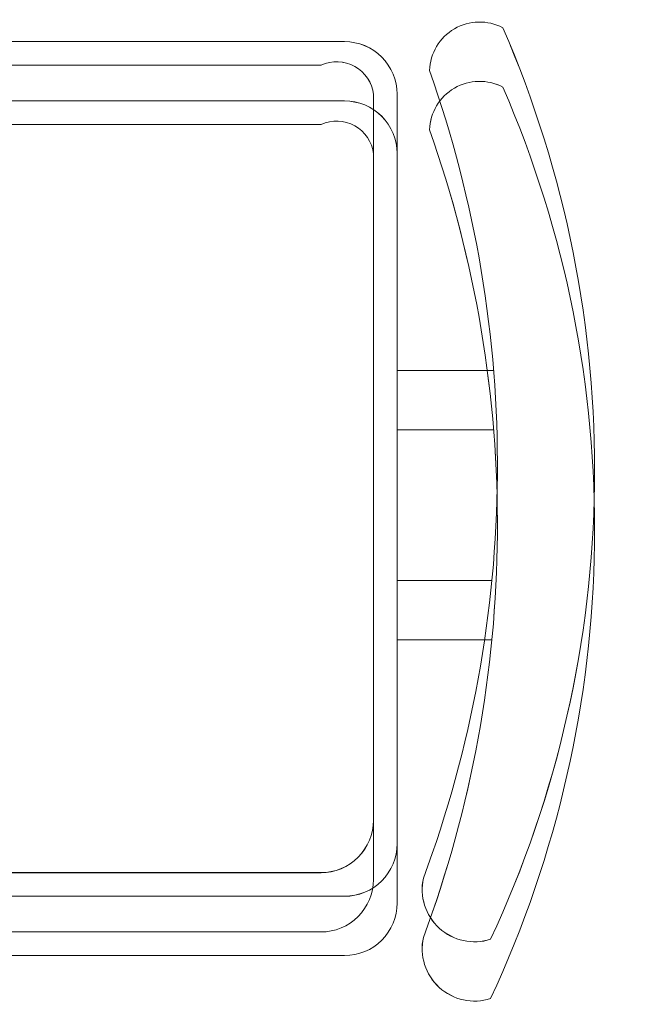
# Model space of a CAD drawing. Units: inches. Extents: x 1885 to 2748, y 783 to 2421.
# Tile 84 of 117: x 2175.64 to 2183.41, y 2082.31 to 2094.85. Entities that reach past the tile are written whole.
import ezdxf

# ---------------------------------------------------------------- set-up
doc = ezdxf.new("R2010")
doc.units = ezdxf.units.IN
doc.layers.add('A-FURN', color=8, linetype='Continuous', lineweight=13)

# ---------------------------------------------------------------- blocks, each defined once
blk = doc.blocks.new('CHAIR-DINING-END')
for points in [[(10.534, 11.861, -0.175809), (10.456, 1.571, 0.578392), (11.313, 0.792, 0.214524), (11.469, 12.407, 0.552014), (10.534, 11.861, -0.065079)], [(10.534, 11.861, -0.175809), (10.456, 1.571, 0.578392), (11.313, 0.791, 0.214524), (11.469, 12.407, 0.552014), (10.534, 11.861, -0.065079)], [(10.121, 11.561, 0.414214), (9.453, 12.229), (0.669, 12.229, 0.414214), (0.001, 11.561), (0.001, 2.008, 0.414214), (0.669, 1.34), (9.453, 1.34, 0.414214), (10.121, 2.008), (10.121, 11.561)], [(10.121, 11.56, 0.414214), (9.453, 12.229), (0.669, 12.229, 0.414214), (0.001, 11.56), (0.001, 2.007, 0.414214), (0.669, 1.339), (9.453, 1.339, 0.414214), (10.121, 2.007), (10.121, 11.56)], [(10.534, 11.106, -0.175809), (10.456, 0.816, 0.578392), (11.313, 0.036, 0.214524), (11.469, 11.651, 0.552014), (10.534, 11.106, -0.065079)], [(10.534, 11.105, -0.175809), (10.456, 0.815, 0.578392), (11.313, 0.036, 0.214524), (11.469, 11.651, 0.552014), (10.534, 11.105, -0.065079)], [(10.121, 10.805, 0.414214), (9.453, 11.474), (0.669, 11.474, 0.414214), (0.001, 10.805), (0.001, 1.252, 0.414214), (0.669, 0.584), (9.453, 0.584, 0.414214), (10.121, 1.252), (10.121, 10.805)], [(10.121, 10.805, 0.414214), (9.453, 11.473), (0.669, 11.473, 0.414214), (0.001, 10.805), (0.001, 1.252, 0.414214), (0.669, 0.584), (9.453, 0.584, 0.414214), (10.121, 1.252), (10.121, 10.805)], [(10.121, 5.363), (11.329, 5.363, -0.064759)], [(10.121, 5.363), (11.329, 5.363, -0.064759)], [(10.121, 4.608), (11.329, 4.608, -0.064759)], [(10.121, 4.607), (11.329, 4.607, -0.064759)]]:
    blk.add_lwpolyline(points, format="xyb")
for points in [[(9.82, 11.557), (9.82, 2.309, -0.414214), (9.152, 1.641), (0.97, 1.641, -0.414214), (0.302, 2.309), (0.302, 11.557, -0.512069), (0.97, 11.928), (9.152, 11.928, -0.512069)], [(9.82, 11.556), (9.82, 2.309, -0.414214), (9.152, 1.64), (0.97, 1.64, -0.414214), (0.302, 2.309), (0.302, 11.556, -0.512069), (0.97, 11.928), (9.152, 11.928, -0.512069)], [(9.82, 10.801), (9.82, 1.553, -0.414214), (9.152, 0.885), (0.97, 0.885, -0.414214), (0.302, 1.553), (0.302, 10.801, -0.512069), (0.97, 11.172), (9.152, 11.172, -0.512069)], [(9.82, 10.801), (9.82, 1.553, -0.414214), (9.152, 0.885), (0.97, 0.885, -0.414214), (0.302, 1.553), (0.302, 10.801, -0.512069), (0.97, 11.172), (9.152, 11.172, -0.512069)]]:
    blk.add_lwpolyline(points, format="xyb", close=True)
for points in [[(11.351, 8.037), (10.121, 8.037)], [(11.351, 8.037), (10.121, 8.037)], [(11.351, 7.282), (10.121, 7.282)], [(11.351, 7.281), (10.121, 7.281)]]:
    blk.add_lwpolyline(points)

msp = doc.modelspace()

# ---------------------------------------------------------------- block references
at = {"layer": 'A-FURN'}
msp.add_blockref('CHAIR-DINING-END', (2170.325, 2082.344), dxfattribs=at)

doc.saveas('drawing.dxf')
